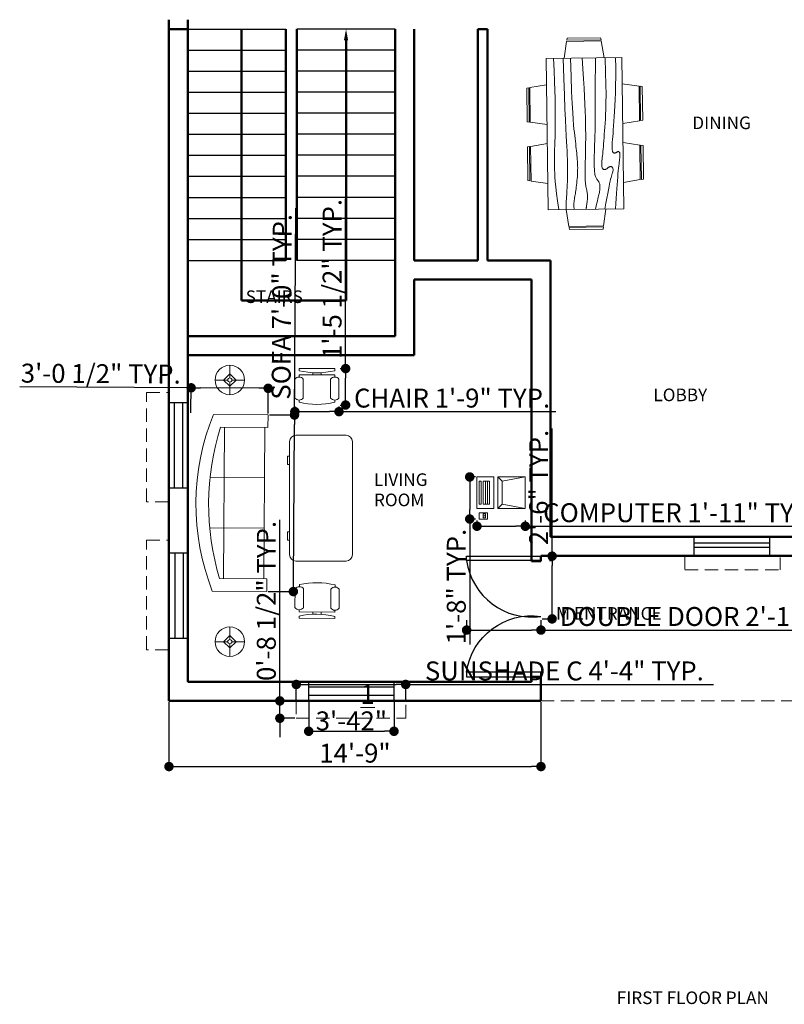
# Model space of a CAD drawing. Units: inches. Extents: x 2050 to 6806, y 2092 to 5743.
# Tile 4 of 8: x 3019 to 3382, y 2203 to 2671. Entities that reach past the tile are written whole.
import ezdxf

# ---------------------------------------------------------------- set-up
doc = ezdxf.new("R2010")
doc.units = ezdxf.units.IN
doc.linetypes.add('HIDDEN', pattern=[9.525, 6.35, -3.175])
for name, color, linetype, lineweight in [('A-ANNO-DIMS', 2, 'Continuous', 18), ('A-ANNO-TEXT', 7, 'Continuous', 25), ('A-AREA-IDEN', 7, 'Continuous', 18), ('A-DOOR', 2, 'Continuous', 25), ('A-FLOR-OVHD', 30, 'HIDDEN', 18), ('A-FLOR-STRS', 3, 'Continuous', 25), ('A-FURN', 5, 'Continuous', 18), ('A-GLAZ', 6, 'Continuous', 25), ('A-WALL', 7, 'Continuous', 50)]:
    doc.layers.add(name, color=color, linetype=linetype, lineweight=lineweight)
doc.styles.get("Standard").update_dxf_attribs({"font": 'arial.ttf'})
doc.dimstyles.new('ISO-25', dxfattribs={"dimtxt": 9, "dimasz": 4.5, "dimexe": 1.25, "dimexo": 0.625, "dimtad": 1, "dimdec": 1, "dimlunit": 4, "dimtxsty": 'Standard', "dimblk": 'DOT', "dimcen": 2.5, "dimadec": 0, "dimazin": 0, "dimtfac": 1, "dimtdec": 1, "dimtmove": 0, "dimatfit": 3, "dimldrblk": 'ARCHTICK', "dimfxl": 1, "dimarcsym": 0})

# ---------------------------------------------------------------- blocks, each defined once
blk = doc.blocks.new('Dining Set - 36 x 72 in.')
for p, q in [((-22.2343, 26.00059), (-23.4847, 17.99762)), ((-22.2304, 26), (-5.7608, 26)), ((-22, 27.5), (-22.1562, 26.50042)), ((-5.8416, 26.5), (-22.1534, 26.5)), ((-22, 27.5), (-6, 27.5)), ((-5.8437, 26.49966), (-6, 27.5)), ((-4.5152, 17.99762), (-5.7655, 25.99926)), ((5.7657, 26.00059), (4.5153, 17.99762)), ((5.7696, 26), (22.2392, 26)), ((6, 27.5), (5.8438, 26.50042)), ((22.1584, 26.5), (5.8466, 26.5)), ((6, 27.5), (22, 27.5)), ((22.1563, 26.49966), (22, 27.5)), ((23.4848, 17.99762), (22.2345, 25.99926)), ((36, 18), (-36, 18)), ((-36, 18), (-36, -18)), ((36, -18), (36, 18)), ((-44.0006, 8.23428), (-35.9976, 9.48474)), ((44.0006, 8.23428), (35.9976, 9.48474)), ((-45.5, 8), (-44.5004, 8.15617)), ((-45.5, 8), (-45.5, -8)), ((-44.5, -8.15843), (-44.5, 8.15338)), ((-44, 8.23041), (-44, -8.23915)), ((44, 8.23041), (44, -8.23915)), ((44.5, -8.15843), (44.5, 8.15338)), ((45.5, 8), (44.5005, 8.15617)), ((45.5, 8), (45.5, -8)), ((-44.4997, -8.15631), (-45.5, -8)), ((-35.9976, -9.48476), (-43.9993, -8.2345)), ((35.9976, -9.48476), (43.9993, -8.2345)), ((44.4997, -8.15631), (45.5, -8)), ((-36, -18), (36, -18)), ((-22.2343, -26.0006), (-23.4847, -17.99762)), ((-4.5152, -17.99762), (-5.7655, -25.99928)), ((5.7657, -26.0006), (4.5153, -17.99762)), ((23.4848, -17.99762), (22.2345, -25.99928)), ((-22.2304, -26), (-5.7608, -26)), ((-22, -27.5), (-22.1562, -26.50044)), ((-5.8416, -26.5), (-22.1534, -26.5)), ((-22, -27.5), (-6, -27.5)), ((-5.8437, -26.49967), (-6, -27.5)), ((5.7696, -26), (22.2392, -26)), ((6, -27.5), (5.8438, -26.50044)), ((22.1584, -26.5), (5.8466, -26.5)), ((6, -27.5), (22, -27.5)), ((22.1563, -26.49967), (22, -27.5))]:
    blk.add_line(p, q)
for points in [[(-36, 15), (-31.1772, 14.97754), (-26.8079, 14.91406), (-22.8538, 14.81543), (-19.276, 14.6875), (-16.0362, 14.53613), (-13.0957, 14.36718), (-10.4159, 14.18652), (-7.9583, 14), (-5.6904, 13.81315), (-3.6035, 13.63021), (-1.6954, 13.45508), (0.0365, 13.29166), (1.5945, 13.14388), (2.9811, 13.01562), (4.1988, 12.9108), (5.25, 12.83333), (6.1393, 12.78613), (6.8802, 12.76823), (7.4883, 12.77767), (7.9792, 12.8125), (8.3685, 12.87077), (8.6719, 12.95052), (8.9049, 13.0498), (9.0833, 13.16666), (9.2205, 13.29899), (9.3216, 13.44401), (9.3895, 13.59879), (9.4271, 13.76041), (9.4373, 13.92594), (9.4232, 14.09245), (9.3875, 14.257), (9.3333, 14.41666), (9.2638, 14.56917), (9.1836, 14.71484), (9.0975, 14.85465), (9.0104, 14.98958), (8.9272, 15.1206), (8.8529, 15.2487), (8.7922, 15.37483), (8.75, 15.5), (8.7305, 15.62467), (8.7344, 15.74739), (8.7617, 15.86621), (8.8125, 15.97916), (8.8867, 16.08431), (8.9844, 16.17968), (9.1055, 16.26334), (9.25, 16.33333), (9.4189, 16.38802), (9.6172, 16.42708), (9.8506, 16.45052), (10.125, 16.45833), (10.4463, 16.45052), (10.8203, 16.42708), (11.2529, 16.38802), (11.75, 16.33333), (12.3184, 16.26318), (12.9694, 16.17838), (13.7151, 16.07991), (14.5677, 15.96875), (15.5395, 15.84586), (16.6426, 15.71224), (17.8893, 15.56884), (19.2917, 15.41666), (20.859, 15.25667), (22.5879, 15.08984), (24.4721, 14.91715), (26.5052, 14.73958), (28.6809, 14.5581), (30.9929, 14.3737), (33.4347, 14.18733), (36, 14)], [(-36, 10), (-28.9766, 10.14274), (-23.1725, 10.20442), (-18.4241, 10.19775), (-14.5677, 10.13541), (-11.4399, 10.03011), (-8.877, 9.89453), (-6.7154, 9.74137), (-4.7917, 9.58333), (-2.9698, 9.43082), (-1.2246, 9.28515), (0.4415, 9.14534), (2.026, 9.01041), (3.5266, 8.87939), (4.9408, 8.7513), (6.266, 8.62516), (7.5, 8.5), (8.6411, 8.37549), (9.6914, 8.2539), (10.6538, 8.13818), (11.5312, 8.03125), (12.3267, 7.93603), (13.043, 7.85547), (13.6831, 7.79248), (14.25, 7.75), (14.7471, 7.7303), (15.1797, 7.73307), (15.5537, 7.75732), (15.875, 7.80208), (16.1494, 7.86637), (16.3828, 7.94922), (16.5811, 8.04964), (16.75, 8.16666), (16.8944, 8.29915), (17.0143, 8.44531), (17.1089, 8.60319), (17.1771, 8.77083), (17.218, 8.94629), (17.2305, 9.1276), (17.2137, 9.31282), (17.1667, 9.5), (17.0895, 9.6875), (16.987, 9.875), (16.8649, 10.0625), (16.7292, 10.25), (16.5856, 10.4375), (16.4401, 10.625), (16.2985, 10.8125), (16.1667, 11), (16.05, 11.18733), (15.9518, 11.3737), (15.8752, 11.5581), (15.8229, 11.73958), (15.798, 11.91715), (15.8034, 12.08984), (15.842, 12.25667), (15.9167, 12.41666), (16.0295, 12.56836), (16.1784, 12.70833), (16.3605, 12.83268), (16.5729, 12.9375), (16.8127, 13.01888), (17.0768, 13.07291), (17.3625, 13.0957), (17.6667, 13.08333), (17.9894, 13.03312), (18.3418, 12.94726), (18.7382, 12.82918), (19.1927, 12.68229), (19.7195, 12.51001), (20.3327, 12.31575), (21.0465, 12.10294), (21.875, 11.875), (22.8357, 11.63354), (23.959, 11.37304), (25.2786, 11.08618), (26.8282, 10.76562), (28.6414, 10.40405), (30.752, 9.99414), (33.1936, 9.52856), (36, 9)], [(-36, 5.5), (-30.7157, 5.3348), (-26.069, 5.20963), (-21.9946, 5.11767), (-18.4271, 5.05208), (-15.3009, 5.00602), (-12.5508, 4.97265), (-10.1112, 4.94515), (-7.9167, 4.91666), (-5.909, 4.88167), (-4.0586, 4.83984), (-2.3429, 4.79215), (-0.7396, 4.73958), (0.7739, 4.6831), (2.22, 4.6237), (3.6213, 4.56233), (5, 4.5), (6.373, 4.43782), (7.7344, 4.3776), (9.0723, 4.32129), (10.375, 4.27083), (11.6309, 4.22819), (12.8281, 4.19531), (13.9551, 4.17415), (15, 4.16666), (15.954, 4.17448), (16.819, 4.19791), (17.6001, 4.23698), (18.3021, 4.29166), (18.9299, 4.36198), (19.4883, 4.44791), (19.9823, 4.54948), (20.4167, 4.66666), (20.7969, 4.79899), (21.1302, 4.94401), (21.4245, 5.09879), (21.6875, 5.26041), (21.9271, 5.42594), (22.1511, 5.59245), (22.3672, 5.757), (22.5834, 5.91666), (22.8065, 6.06868), (23.0404, 6.21093), (23.2879, 6.34147), (23.5521, 6.45833), (23.8358, 6.55957), (24.142, 6.64323), (24.4735, 6.70735), (24.8334, 6.75), (25.2235, 6.76969), (25.642, 6.76692), (26.0858, 6.74267), (26.5521, 6.69791), (27.0379, 6.63362), (27.5404, 6.55078), (28.0565, 6.45036), (28.5834, 6.33333), (29.1242, 6.19987), (29.7071, 6.04687), (30.3661, 5.87044), (31.1354, 5.66666), (32.0493, 5.43164), (33.142, 5.16146), (34.4475, 4.85221), (36, 4.5)], [(-36, -1), (-30.7915, -0.6591), (-26.0195, -0.38216), (-21.6519, -0.16284), (-17.6563, 0.00521), (-14.0005, 0.12833), (-10.6523, 0.21289), (-7.5796, 0.26522), (-4.75, 0.29166), (-2.134, 0.29793), (0.2878, 0.28711), (2.5317, 0.26163), (4.6146, 0.22396), (6.5529, 0.17651), (8.3633, 0.12174), (10.0623, 0.06209), (11.6667, 0), (13.1899, -0.06201), (14.6341, -0.1211), (15.9982, -0.17432), (17.2813, -0.21875), (18.4823, -0.25147), (19.6003, -0.26953), (20.6343, -0.27002), (21.5834, -0.25), (22.4481, -0.20768), (23.2357, -0.14584), (23.9549, -0.06836), (24.6146, 0.02083), (25.2235, 0.11784), (25.7904, 0.21875), (26.3241, 0.31966), (26.8334, 0.41666), (27.3265, 0.50618), (27.8099, 0.58593), (28.2894, 0.65397), (28.7709, 0.70833), (29.2601, 0.74707), (29.763, 0.76823), (30.2855, 0.76985), (30.8334, 0.75), (31.4088, 0.70784), (31.9994, 0.64713), (32.589, 0.57275), (33.1615, 0.48958), (33.7008, 0.4025), (34.1908, 0.3164), (34.6153, 0.23616), (34.9584, 0.16666), (35.2099, 0.11165), (35.3848, 0.07031), (35.504, 0.04069), (35.5886, 0.02083), (35.6594, 0.00879), (35.7377, 0.0026), (35.8442, 0.00032), (36, 0)], [(-36, -6.5), (-27.1843, -6.31267), (-20.084, -6.1263), (-14.469, -5.9419), (-10.1094, -5.76042), (-6.7752, -5.58285), (-4.2363, -5.41016), (-2.2629, -5.24333), (-0.625, -5.08334), (0.8708, -4.93099), (2.2715, -4.78646), (3.5872, -4.64974), (4.8281, -4.52084), (6.0046, -4.39974), (7.127, -4.28646), (8.2053, -4.18099), (9.25, -4.08334), (10.2705, -3.99382), (11.2734, -3.91407), (12.2647, -3.84603), (13.25, -3.79167), (14.2354, -3.75293), (15.2266, -3.73177), (16.2295, -3.73015), (17.25, -3.75), (18.2912, -3.79248), (19.3451, -3.85547), (20.4009, -3.93604), (21.4479, -4.03125), (22.4754, -4.13819), (23.4727, -4.25391), (24.4289, -4.37549), (25.3334, -4.5), (26.1785, -4.62492), (26.9694, -4.74935), (27.7145, -4.87281), (28.4219, -4.99479), (29.1, -5.11483), (29.7572, -5.23242), (30.4016, -5.34709), (31.0417, -5.45834), (31.6837, -5.56437), (32.3262, -5.65821), (32.9658, -5.73153), (33.599, -5.77604), (34.2224, -5.78345), (34.8327, -5.74545), (35.4264, -5.65373), (36, -5.5)], [(-36, -10), (-26.4022, -9.81299), (-18.4675, -9.62891), (-11.9839, -9.45069), (-6.7396, -9.28125), (-2.5226, -9.12354), (0.8789, -8.98047), (3.6769, -8.85498), (6.0833, -8.75), (8.2767, -8.66765), (10.3021, -8.60677), (12.1712, -8.56543), (13.8958, -8.54167), (15.4876, -8.53353), (16.9583, -8.53907), (18.3197, -8.55632), (19.5834, -8.58334), (20.7616, -8.61841), (21.8685, -8.66081), (22.9188, -8.71004), (23.9271, -8.76563), (24.9081, -8.82707), (25.8763, -8.89388), (26.8465, -8.96558), (27.8334, -9.04167), (28.8474, -9.12118), (29.8828, -9.20117), (30.93, -9.27824), (31.9792, -9.34896), (33.0205, -9.40991), (34.0443, -9.45768), (35.0407, -9.48885), (36, -9.5)], [(-36, -14.5), (-30.0881, -14.33513), (-25.0332, -14.21224), (-20.7312, -14.12647), (-17.0781, -14.07292), (-13.97, -14.04671), (-11.3027, -14.04297), (-8.9724, -14.05681), (-6.875, -14.08334), (-4.9224, -14.11833), (-3.0905, -14.16016), (-1.3709, -14.20785), (0.2448, -14.26042), (1.7647, -14.3169), (3.1973, -14.3763), (4.5507, -14.43767), (5.8333, -14.5), (7.0554, -14.5621), (8.235, -14.62175), (9.3922, -14.67652), (10.5469, -14.72396), (11.7192, -14.76164), (12.929, -14.78711), (14.1965, -14.79794), (15.5417, -14.79167), (16.9933, -14.76424), (18.6152, -14.70508), (20.4804, -14.60197), (22.6615, -14.44271), (25.2312, -14.21509), (28.2624, -13.9069), (31.8277, -13.50594), (36, -13)]]:
    blk.add_lwpolyline(points)
blk = doc.blocks.new('Sofa - Roundback 7 ft.')
for p, q in [((-12.00002, -32.4421), (-12.00003, -6.5971)), ((11.99997, -32.4421), (11.99998, -6.5971)), ((-36.000027, -34), (-36.000027, -11.4696)), ((-35.999844, -13.3819), (35.9998, -13.3819)), ((35.99998, -34), (35.99998, -11.4696)), ((-36.000027, -32.4421), (35.99998, -32.4421))]:
    blk.add_line(p, q)
for points in [[(-36.000027, -34), (-42.000027, -34), (-42.000027, -8)], [(41.99998, -8), (41.99998, -34), (35.99998, -34)]]:
    blk.add_lwpolyline(points)
for centre, radius, start, end in [((0, -114.25), 114.25, 68.43141, 111.5686), ((-0.00001, -127.1968), 121.1968, 72.72033, 107.2797)]:
    blk.add_arc(centre, radius, start, end)
blk = doc.blocks.new('Desk - 30 x 60 in.')
for p, q in [((-26.999995, 0), (26.999995, 0)), ((-29.999995, -27), (-29.999995, -3)), ((29.999995, -3), (29.999995, -27)), ((26.999995, -30), (-26.999995, -30)), ((-20.000005, -30), (-20.000005, -31)), ((-20.000005, -31), (-16.000005, -31)), ((-16.000005, -31), (-16.000005, -30)), ((15.999995, -31), (15.999995, -30)), ((19.999995, -31), (15.999995, -31)), ((19.999995, -30), (19.999995, -31))]:
    blk.add_line(p, q)
for centre, start, end in [((-26.499995, -3.5), 98.1301, 171.8699), ((26.499995, -3.5), 8.130102, 81.8699), ((-26.499995, -26.5), 188.1301, 261.8699), ((26.499995, -26.5), 278.1301, 351.8699)]:
    blk.add_arc(centre, 3.535534, start, end)
blk = doc.blocks.new('Chair - Desk')
for p, q in [((-8.5, 0), (-8.5, -1)), ((-8.5, 0), (8.5, 0)), ((8.5, 0), (8.5, -1)), ((-8.5, -3), (-8.5, -4)), ((-8.5, -3), (8.5, -3)), ((-2, -3), (-2, -1.9355)), ((2, -1.9576), (2, -3)), ((8.5, -3), (8.5, -4)), ((-10.5, -5), (-10.5, -14)), ((-6.5, -14), (-6.5, -5)), ((6.5, -5), (6.5, -14)), ((10.5, -14), (10.5, -5)), ((-8.5, -15), (-8.5, -16)), ((8.5, -15), (8.5, -16))]:
    blk.add_line(p, q)
for centre, radius, start, end in [((-8.5, -6.5), 2.5, 36.8699, 143.1301), ((0, 34.625), 36.625, 256.5803, 283.4197), ((8.5, -6.5), 2.5, 36.8699, 143.1301), ((-8.5, -12.5), 2.5, 216.8699, 323.1301), ((8.5, -12.5), 2.5, 216.8699, 323.1301), ((0, 19.625), 36.625, 256.5803, 283.4197)]:
    blk.add_arc(centre, radius, start, end)
blk = doc.blocks.new('Lamp - Table')
for p, q in [((0, 7), (0, 1)), ((-1, 0), (-7, 0)), ((0, 3), (-3, 0)), ((-3, 0), (0, -3)), ((3, 0), (0, 3)), ((0, -3), (3, 0)), ((1, 0), (7, 0)), ((0, -1), (0, -7))]:
    blk.add_line(p, q)
for radius in [7, 1]:
    blk.add_circle((0, 0), radius)
blk = doc.blocks.new('Computer Terminal')
for p, q in [((-10, 11.5), (5, 11.5)), ((-8, 0.5), (-10, 11.5)), ((-10, -1.5), (-10, 11.5)), ((5, 11.5), (3, 0.5)), ((5, 11.5), (5, -1.5)), ((-10, -1.5), (-8, 0.5)), ((3, 0.5), (-8, 0.5)), ((3, 0.5), (5, -1.5)), ((5, -1.5), (-10, -1.5)), ((-10, -11.5), (-10, -3.5)), ((-10, -3.5), (5, -3.5)), ((5, -3.5), (5, -11.5)), ((-8, -5.5), (-8, -8.5)), ((3, -5.5), (-8, -5.5)), ((3, -6.5), (-8, -6.5)), ((-8, -7.5), (3, -7.5)), ((-8, -8.5), (3, -8.5)), ((3, -8.5), (3, -5.5)), ((10, -6.5), (7, -6.5)), ((7, -6.5), (7, -10.5)), ((9.5, -7.5), (7.5, -7.5)), ((7.5, -7.5), (7.5, -8.5)), ((7.5, -8.5), (9.5, -8.5)), ((8.5, -7.5), (8.5, -8.5)), ((9.5, -8.5), (9.5, -7.5)), ((10, -10.5), (10, -6.5)), ((5, -11.5), (-10, -11.5)), ((-8, -9.5), (-8, -10.5)), ((3, -9.5), (-8, -9.5)), ((-8, -10.5), (3, -10.5)), ((3, -10.5), (3, -9.5)), ((7, -10.5), (10, -10.5))]:
    blk.add_line(p, q)
blk = doc.blocks.new('_Dot')
at = {"color": 0, "linetype": 'ByBlock', "lineweight": -2}
blk.add_line((-0.5, 0), (-1, 0), dxfattribs=at)
at = {"color": 0, "linetype": 'ByBlock', "const_width": 0.5}
blk.add_lwpolyline([(-0.25, 0, 1), (0.25, 0, 1)], format="xyb", close=True, dxfattribs=at)
blk = doc.blocks.new('*D41')
at = {"layer": 'A-ANNO-DIMS', "color": 0, "lineweight": -2, "transparency": 16777216}
for p, q in [((3156.16, 2346.7), (3156.16, 2331.62)), ((3196.75, 2346.7), (3196.75, 2331.62)), ((3160.66, 2332.87), (3192.25, 2332.87))]:
    blk.add_line(p, q, dxfattribs=at)
at = {"layer": 'Defpoints', "color": 0, "transparency": 16777216}
for p in [(3156.16, 2347.33), (3196.75, 2347.32), (3196.75, 2332.87)]:
    blk.add_point(p, dxfattribs=at)
at = {"layer": 'A-ANNO-DIMS', "color": 0, "lineweight": -2, "transparency": 16777216, "xscale": 4.5, "yscale": 4.5, "zscale": 4.5, "rotation": 180}
blk.add_blockref('_Dot', (3156.16, 2332.87), dxfattribs=at)
at = {"layer": 'A-ANNO-DIMS', "color": 0, "lineweight": -2, "transparency": 16777216, "xscale": 4.5, "yscale": 4.5, "zscale": 4.5}
blk.add_blockref('_Dot', (3196.75, 2332.87), dxfattribs=at)
at = {"layer": 'A-ANNO-DIMS', "color": 0, "transparency": 16777216, "insert": (3176.46, 2344.12), "char_height": 9, "attachment_point": 5}
blk.add_mtext('3\'-4{\\H1x;\\S1/2;}"', dxfattribs=at)
blk = doc.blocks.new('_ArchTick')
at = {"color": 0, "linetype": 'ByBlock', "const_width": 0.15}
blk.add_lwpolyline([(-0.5, -0.5), (0.5, 0.5)], dxfattribs=at)
blk = doc.blocks.new('*D42')
at = {"layer": 'A-ANNO-DIMS', "color": 0, "lineweight": -2, "transparency": 16777216}
for p, q in [((3089.67, 2346.7), (3089.67, 2314.85)), ((3266.67, 2346.7), (3266.67, 2314.85)), ((3094.17, 2316.1), (3262.17, 2316.1))]:
    blk.add_line(p, q, dxfattribs=at)
at = {"layer": 'Defpoints', "color": 0, "transparency": 16777216}
for p in [(3089.67, 2347.33), (3266.67, 2347.33), (3266.67, 2316.1)]:
    blk.add_point(p, dxfattribs=at)
at = {"layer": 'A-ANNO-DIMS', "color": 0, "lineweight": -2, "transparency": 16777216, "xscale": 4.5, "yscale": 4.5, "zscale": 4.5, "rotation": 180}
blk.add_blockref('_Dot', (3089.67, 2316.1), dxfattribs=at)
at = {"layer": 'A-ANNO-DIMS', "color": 0, "lineweight": -2, "transparency": 16777216, "xscale": 4.5, "yscale": 4.5, "zscale": 4.5}
blk.add_blockref('_Dot', (3266.67, 2316.1), dxfattribs=at)
at = {"layer": 'A-ANNO-DIMS', "color": 0, "transparency": 16777216, "insert": (3178.17, 2321.32), "char_height": 9, "attachment_point": 5}
blk.add_mtext('14\'-9"', dxfattribs=at)
blk = doc.blocks.new('DOOR-750')
blk.add_lwpolyline([(28.97, 0), (26.83, 0), (26.83, 35.38), (28.97, 35.38)], close=True)
blk.add_arc((31.25, 4.42), 31.27, 98.1233, 188.1233)
blk = doc.blocks.new('DOOR-DOUBLE')
blk.add_lwpolyline([(35.38, 28.96), (35.38, 26.82), (0, 26.82), (0, 28.96)], close=True)
blk.add_lwpolyline([(35.38, 28.96), (35.38, 26.82), (0, 26.82), (0, 28.96)], close=True)
blk.add_arc((30.96, 31.24), 31.27, 188.1233, 278.1233)
blk.add_arc((30.96, 31.24), 31.27, 188.1233, 278.1233)
blk = doc.blocks.new('WIN-1050')
for p, q in [((0, 40.58), (9, 40.58)), ((2.5, 0), (2.5, 40.58)), ((6.5, 0), (6.5, 40.58)), ((0, 0), (9, 0))]:
    blk.add_line(p, q)
blk = doc.blocks.new('WIN-900')
for p, q in [((0, 9), (0, 0)), ((36, 5.99), (0, 5.99)), ((36, 9), (36, 0)), ((36, 3.99), (0, 3.99)), ((36, 3.99), (0, 3.99))]:
    blk.add_line(p, q)
blk = doc.blocks.new('SUNSHADE-A')
for p, q in [((0, 52.08), (10.45, 52.08)), ((10.45, 52.08), (10.45, 0)), ((10.45, 0), (0, 0))]:
    blk.add_line(p, q)
blk = doc.blocks.new('SUNSHADE-C')
for p, q in [((0, 8.26), (0, 0)), ((52.07, 0), (52.07, 8.25)), ((0, 0), (52.07, 0))]:
    blk.add_line(p, q)
blk = doc.blocks.new('*D77')
at = {"layer": 'A-ANNO-DIMS', "color": 0, "lineweight": -2, "transparency": 16777216}
for p, q in [((3231.3, 2385.71), (3231.3, 2379.77)), ((3266.67, 2385.71), (3266.67, 2379.77)), ((3235.8, 2381.02), (3262.17, 2381.02)), ((3266.67, 2381.02), (3451.21, 2381.02))]:
    blk.add_line(p, q, dxfattribs=at)
at = {"layer": 'Defpoints', "color": 0, "transparency": 16777216}
for p in [(3231.3, 2386.33), (3266.67, 2386.33), (3266.67, 2381.02)]:
    blk.add_point(p, dxfattribs=at)
at = {"layer": 'A-ANNO-DIMS', "color": 0, "lineweight": -2, "transparency": 16777216, "xscale": 4.5, "yscale": 4.5, "zscale": 4.5, "rotation": 180}
blk.add_blockref('_Dot', (3231.3, 2381.02), dxfattribs=at)
at = {"layer": 'A-ANNO-DIMS', "color": 0, "lineweight": -2, "transparency": 16777216, "xscale": 4.5, "yscale": 4.5, "zscale": 4.5}
blk.add_blockref('_Dot', (3266.67, 2381.02), dxfattribs=at)
at = {"layer": 'A-ANNO-DIMS', "color": 0, "transparency": 16777216, "insert": (3361.19, 2386.31), "char_height": 9, "attachment_point": 5}
blk.add_mtext('DOUBLE DOOR 2\'-11 1/2" TYP.', dxfattribs=at)
blk = doc.blocks.new('*D78')
at = {"layer": 'A-ANNO-DIMS', "color": 0, "lineweight": -2, "transparency": 16777216}
for p, q in [((3271.98, 2416.18), (3271.98, 2476.94)), ((3267.3, 2416.18), (3273.23, 2416.18)), ((3271.98, 2390.83), (3271.98, 2411.68)), ((3267.3, 2386.33), (3273.23, 2386.33))]:
    blk.add_line(p, q, dxfattribs=at)
at = {"layer": 'Defpoints', "color": 0, "transparency": 16777216}
for p in [(3266.67, 2416.18), (3271.98, 2416.18), (3266.67, 2386.33)]:
    blk.add_point(p, dxfattribs=at)
at = {"layer": 'A-ANNO-DIMS', "color": 0, "lineweight": -2, "transparency": 16777216, "xscale": 4.5, "yscale": 4.5, "zscale": 4.5}
for p, rotation in [((3271.98, 2416.18), 90), ((3271.98, 2386.33), 270)]:
    blk.add_blockref('_Dot', p, dxfattribs=dict(at, rotation=rotation))
at = {"layer": 'A-ANNO-DIMS', "color": 0, "transparency": 16777216, "insert": (3266.76, 2448.81), "char_height": 9, "attachment_point": 5, "rotation": 90}
blk.add_mtext('2\'-6" TYP.', dxfattribs=at)
blk = doc.blocks.new('*D83')
at = {"layer": 'A-ANNO-DIMS', "color": 0, "lineweight": -2, "transparency": 16777216}
for p, q in [((3150.25, 2347.95), (3150.25, 2356.39)), ((3202.32, 2347.95), (3202.32, 2356.39)), ((3154.75, 2355.14), (3197.82, 2355.14)), ((3202.32, 2355.14), (3348.82, 2355.14))]:
    blk.add_line(p, q, dxfattribs=at)
at = {"layer": 'Defpoints', "color": 0, "transparency": 16777216}
for p in [(3202.32, 2355.14), (3150.25, 2347.33), (3202.32, 2347.33)]:
    blk.add_point(p, dxfattribs=at)
at = {"layer": 'A-ANNO-DIMS', "color": 0, "lineweight": -2, "transparency": 16777216, "xscale": 4.5, "yscale": 4.5, "zscale": 4.5, "rotation": 180}
blk.add_blockref('_Dot', (3150.25, 2355.14), dxfattribs=at)
at = {"layer": 'A-ANNO-DIMS', "color": 0, "lineweight": -2, "transparency": 16777216, "xscale": 4.5, "yscale": 4.5, "zscale": 4.5}
blk.add_blockref('_Dot', (3202.32, 2355.14), dxfattribs=at)
at = {"layer": 'A-ANNO-DIMS', "color": 0, "transparency": 16777216, "insert": (3277.82, 2360.42), "char_height": 9, "attachment_point": 5}
blk.add_mtext('SUNSHADE C 4\'-4" TYP.', dxfattribs=at)
blk = doc.blocks.new('*D84')
at = {"layer": 'A-ANNO-DIMS', "color": 0, "lineweight": -2, "transparency": 16777216}
for p, q in [((3142.44, 2351.83), (3142.44, 2433.41)), ((3149.63, 2347.33), (3141.19, 2347.33)), ((3142.44, 2339.07), (3142.44, 2347.33)), ((3149.63, 2339.07), (3141.19, 2339.07)), ((3142.44, 2334.57), (3142.44, 2330.07))]:
    blk.add_line(p, q, dxfattribs=at)
at = {"layer": 'Defpoints', "color": 0, "transparency": 16777216}
for p in [(3142.44, 2347.33), (3150.25, 2347.33), (3150.25, 2339.07)]:
    blk.add_point(p, dxfattribs=at)
at = {"layer": 'A-ANNO-DIMS', "color": 0, "lineweight": -2, "transparency": 16777216, "xscale": 4.5, "yscale": 4.5, "zscale": 4.5}
for p, rotation in [((3142.44, 2347.33), 270), ((3142.44, 2339.07), 90)]:
    blk.add_blockref('_Dot', p, dxfattribs=dict(at, rotation=rotation))
at = {"layer": 'A-ANNO-DIMS', "color": 0, "transparency": 16777216, "insert": (3137.16, 2394.87), "char_height": 9, "attachment_point": 5, "rotation": 90}
blk.add_mtext('0\'-8 1/2" TYP.', dxfattribs=at)
blk = doc.blocks.new('*D89')
at = {"layer": 'A-ANNO-DIMS', "color": 0, "lineweight": -2, "transparency": 16777216}
for p, q in [((3149.58, 2487.43), (3149.58, 2483.65)), ((3170.58, 2487.43), (3170.58, 2483.65)), ((3154.08, 2484.9), (3166.08, 2484.9)), ((3170.58, 2484.9), (3273.7, 2484.9))]:
    blk.add_line(p, q, dxfattribs=at)
at = {"layer": 'Defpoints', "color": 0, "transparency": 16777216}
for p in [(3149.58, 2488.05), (3170.58, 2488.05), (3170.58, 2484.9)]:
    blk.add_point(p, dxfattribs=at)
at = {"layer": 'A-ANNO-DIMS', "color": 0, "lineweight": -2, "transparency": 16777216, "xscale": 4.5, "yscale": 4.5, "zscale": 4.5, "rotation": 180}
blk.add_blockref('_Dot', (3149.58, 2484.9), dxfattribs=at)
at = {"layer": 'A-ANNO-DIMS', "color": 0, "lineweight": -2, "transparency": 16777216, "xscale": 4.5, "yscale": 4.5, "zscale": 4.5}
blk.add_blockref('_Dot', (3170.58, 2484.9), dxfattribs=at)
at = {"layer": 'A-ANNO-DIMS', "color": 0, "transparency": 16777216, "insert": (3224.39, 2490.18), "char_height": 9, "attachment_point": 5}
blk.add_mtext('CHAIR 1\'-9" TYP.', dxfattribs=at)
blk = doc.blocks.new('*D90')
at = {"layer": 'A-ANNO-DIMS', "color": 0, "lineweight": -2, "transparency": 16777216}
for p, q in [((3173.73, 2505.38), (3173.73, 2586.12)), ((3171.2, 2505.38), (3174.98, 2505.38)), ((3173.73, 2492.55), (3173.73, 2500.88)), ((3171.2, 2488.05), (3174.98, 2488.05))]:
    blk.add_line(p, q, dxfattribs=at)
at = {"layer": 'Defpoints', "color": 0, "transparency": 16777216}
for p in [(3170.58, 2505.38), (3173.73, 2505.38), (3170.58, 2488.05)]:
    blk.add_point(p, dxfattribs=at)
at = {"layer": 'A-ANNO-DIMS', "color": 0, "lineweight": -2, "transparency": 16777216, "xscale": 4.5, "yscale": 4.5, "zscale": 4.5}
for p, rotation in [((3173.73, 2505.38), 90), ((3173.73, 2488.05), 270)]:
    blk.add_blockref('_Dot', p, dxfattribs=dict(at, rotation=rotation))
at = {"layer": 'A-ANNO-DIMS', "color": 0, "transparency": 16777216, "insert": (3168.45, 2548), "char_height": 9, "attachment_point": 5, "rotation": 90}
blk.add_mtext('1\'-5 1/2" TYP.', dxfattribs=at)
blk = doc.blocks.new('*D95')
at = {"layer": 'A-ANNO-DIMS', "color": 0, "lineweight": -2, "transparency": 16777216}
for p, q in [((3149.41, 2483.32), (3150.05, 2581.61)), ((3137.44, 2483.4), (3150.66, 2483.31)), ((3148.89, 2403.82), (3149.38, 2478.82)), ((3136.89, 2399.4), (3150.11, 2399.32))]:
    blk.add_line(p, q, dxfattribs=at)
at = {"layer": 'Defpoints', "color": 0, "transparency": 16777216}
for p in [(3136.81, 2483.41), (3149.41, 2483.32), (3136.26, 2399.41)]:
    blk.add_point(p, dxfattribs=at)
at = {"layer": 'A-ANNO-DIMS', "color": 0, "lineweight": -2, "transparency": 16777216, "xscale": 4.5, "yscale": 4.5, "zscale": 4.5}
for p, rotation in [((3149.41, 2483.32), 89.62659340575084), ((3148.86, 2399.32), 269.6265934057509)]:
    blk.add_blockref('_Dot', p, dxfattribs=dict(at, rotation=rotation))
at = {"layer": 'A-ANNO-DIMS', "color": 0, "transparency": 16777216, "insert": (3144.46, 2534.75), "char_height": 9, "attachment_point": 5, "rotation": 89.6266}
blk.add_mtext('SOFA 7\'-0" TYP.', dxfattribs=at)
blk = doc.blocks.new('*D96')
at = {"layer": 'A-ANNO-DIMS', "color": 0, "lineweight": -2, "transparency": 16777216}
for p, q in [((3100.23, 2496.24), (3018.65, 2496.78)), ((3100.15, 2484.27), (3100.23, 2497.49)), ((3132.39, 2496.03), (3104.73, 2496.21)), ((3136.81, 2484.03), (3136.9, 2497.25))]:
    blk.add_line(p, q, dxfattribs=at)
at = {"layer": 'Defpoints', "color": 0, "transparency": 16777216}
for p in [(3100.23, 2496.24), (3100.14, 2483.64), (3136.81, 2483.41)]:
    blk.add_point(p, dxfattribs=at)
at = {"layer": 'A-ANNO-DIMS', "color": 0, "lineweight": -2, "transparency": 16777216, "xscale": 4.5, "yscale": 4.5, "zscale": 4.5}
for p, rotation in [((3100.23, 2496.24), 179.6265934057506), ((3136.89, 2496), 359.6265934057507)]:
    blk.add_blockref('_Dot', p, dxfattribs=dict(at, rotation=rotation))
at = {"layer": 'A-ANNO-DIMS', "color": 0, "transparency": 16777216, "insert": (3057.22, 2501.81), "char_height": 9, "attachment_point": 5, "rotation": 359.6266}
blk.add_mtext('3\'-0 1/2" TYP.', dxfattribs=at)
blk = doc.blocks.new('*D99')
at = {"layer": 'A-ANNO-DIMS', "color": 0, "lineweight": -2, "transparency": 16777216}
for p, q in [((3236.22, 2433.21), (3236.22, 2429.14)), ((3259.22, 2433.21), (3259.22, 2429.14)), ((3240.72, 2430.39), (3254.72, 2430.39)), ((3259.22, 2430.39), (3402.15, 2430.39))]:
    blk.add_line(p, q, dxfattribs=at)
at = {"layer": 'Defpoints', "color": 0, "transparency": 16777216}
for p in [(3236.22, 2433.84), (3259.22, 2433.84), (3259.22, 2430.39)]:
    blk.add_point(p, dxfattribs=at)
at = {"layer": 'A-ANNO-DIMS', "color": 0, "lineweight": -2, "transparency": 16777216, "xscale": 4.5, "yscale": 4.5, "zscale": 4.5, "rotation": 180}
blk.add_blockref('_Dot', (3236.22, 2430.39), dxfattribs=at)
at = {"layer": 'A-ANNO-DIMS', "color": 0, "lineweight": -2, "transparency": 16777216, "xscale": 4.5, "yscale": 4.5, "zscale": 4.5}
blk.add_blockref('_Dot', (3259.22, 2430.39), dxfattribs=at)
at = {"layer": 'A-ANNO-DIMS', "color": 0, "transparency": 16777216, "insert": (3332.93, 2435.67), "char_height": 9, "attachment_point": 5}
blk.add_mtext('COMPUTER 1\'-11" TYP.', dxfattribs=at)
blk = doc.blocks.new('*D100')
at = {"layer": 'A-ANNO-DIMS', "color": 0, "lineweight": -2, "transparency": 16777216}
for p, q in [((3235.59, 2453.84), (3231.52, 2453.84)), ((3232.77, 2449.34), (3232.77, 2438.34)), ((3235.59, 2433.84), (3231.52, 2433.84)), ((3232.77, 2433.84), (3232.77, 2374.08))]:
    blk.add_line(p, q, dxfattribs=at)
at = {"layer": 'Defpoints', "color": 0, "transparency": 16777216}
for p in [(3236.22, 2453.84), (3232.77, 2433.84), (3236.22, 2433.84)]:
    blk.add_point(p, dxfattribs=at)
at = {"layer": 'A-ANNO-DIMS', "color": 0, "lineweight": -2, "transparency": 16777216, "xscale": 4.5, "yscale": 4.5, "zscale": 4.5}
for p, rotation in [((3232.77, 2453.84), 90), ((3232.77, 2433.84), 270)]:
    blk.add_blockref('_Dot', p, dxfattribs=dict(at, rotation=rotation))
at = {"layer": 'A-ANNO-DIMS', "color": 0, "transparency": 16777216, "insert": (3227.55, 2401.71), "char_height": 9, "attachment_point": 5, "rotation": 90}
blk.add_mtext('1\'-8" TYP.', dxfattribs=at)

msp = doc.modelspace()

# ---------------------------------------------------------------- linework, layer by layer
at = {"layer": 'A-FLOR-OVHD'}
for p, q in [((3335.17, 2416.33), (3335.17, 2409.73)), ((3380.52, 2409.73), (3380.52, 2415.55)), ((3335.17, 2409.73), (3380.52, 2409.73)), ((3266.67, 2347.33), (3446.67, 2347.33))]:
    msp.add_line(p, q, dxfattribs=at)
at = {"layer": 'A-FLOR-STRS'}
for p, q in [((3098.67, 2666.83), (3134.67, 2666.83)), ((3098.67, 2666.83), (3145.36, 2666.83)), ((3197.28, 2666.83), (3150.59, 2666.83)), ((3197.28, 2666.83), (3161.28, 2666.83)), ((3098.67, 2656.83), (3145.36, 2656.83)), ((3197.28, 2656.83), (3150.59, 2656.83)), ((3098.67, 2646.83), (3145.36, 2646.83)), ((3197.28, 2646.83), (3150.59, 2646.83)), ((3098.67, 2636.83), (3145.36, 2636.83)), ((3197.28, 2636.83), (3150.59, 2636.83)), ((3098.67, 2626.83), (3145.36, 2626.83)), ((3197.28, 2626.83), (3150.59, 2626.83)), ((3098.67, 2616.83), (3145.36, 2616.83)), ((3197.28, 2616.83), (3150.59, 2616.83)), ((3098.67, 2606.83), (3145.36, 2606.83)), ((3197.28, 2606.83), (3150.59, 2606.83)), ((3098.67, 2596.83), (3145.36, 2596.83)), ((3197.28, 2596.83), (3150.59, 2596.83)), ((3098.67, 2586.83), (3145.36, 2586.83)), ((3197.28, 2586.83), (3150.59, 2586.83)), ((3098.67, 2576.83), (3145.36, 2576.83)), ((3197.28, 2576.83), (3150.59, 2576.83)), ((3098.67, 2566.83), (3145.36, 2566.83)), ((3197.28, 2566.83), (3150.59, 2566.83)), ((3098.67, 2556.83), (3145.36, 2556.83)), ((3197.28, 2556.83), (3150.59, 2556.83)), ((3098.67, 2520.83), (3145.36, 2520.83))]:
    msp.add_line(p, q, dxfattribs=at)
at = {"layer": 'A-WALL'}
for p, q in [((3089.67, 2671.33), (3089.67, 2347.33)), ((3098.67, 2671.33), (3098.67, 2356.33)), ((3098.67, 2666.83), (3089.67, 2666.83)), ((3124.15, 2537.84), (3124.15, 2666.83)), ((3145.36, 2666.83), (3145.36, 2556.83)), ((3150.59, 2666.83), (3150.59, 2556.83)), ((3197.28, 2666.83), (3197.28, 2520.83)), ((3206.28, 2666.83), (3206.28, 2556.83)), ((3236.67, 2635.96), (3236.67, 2666.83)), ((3236.67, 2666.83), (3241.17, 2666.83)), ((3241.17, 2635.96), (3241.17, 2666.83)), ((3173.93, 2661.55), (3173.93, 2537.84)), ((3236.67, 2556.83), (3236.67, 2635.96)), ((3241.17, 2556.83), (3241.17, 2635.96)), ((3206.28, 2556.83), (3236.67, 2556.83)), ((3241.17, 2556.83), (3262.17, 2556.83)), ((3262.17, 2556.83), (3271.17, 2556.83)), ((3271.17, 2556.83), (3271.17, 2547.83)), ((3206.28, 2547.83), (3262.17, 2547.83)), ((3206.28, 2547.83), (3206.28, 2511.83)), ((3262.17, 2547.83), (3262.17, 2413.83)), ((3271.17, 2547.83), (3271.17, 2425.33)), ((3173.93, 2537.84), (3124.15, 2537.84)), ((3197.28, 2520.83), (3098.67, 2520.83)), ((3206.28, 2511.83), (3098.67, 2511.83)), ((3271.17, 2425.33), (3442.17, 2425.33)), ((3266.67, 2413.83), (3262.17, 2413.83)), ((3266.67, 2416.33), (3446.67, 2416.33)), ((3266.67, 2416.33), (3266.67, 2413.83)), ((3271.17, 2416.33), (3271.17, 2413.83)), ((3098.67, 2356.33), (3262.17, 2356.33)), ((3262.17, 2358.83), (3262.17, 2356.33)), ((3262.17, 2358.83), (3266.67, 2358.83)), ((3266.67, 2358.83), (3266.67, 2347.33)), ((3089.67, 2347.33), (3266.67, 2347.33))]:
    msp.add_line(p, q, dxfattribs=at)
msp.add_lwpolyline([(3173.93, 2666.83, 0, 2, 0), (3173.93, 2661.55, 2, 2, 0)], format="xyseb", dxfattribs=at)

# ---------------------------------------------------------------- block references
at = {"layer": 'A-DOOR'}
msp.add_blockref('DOOR-DOUBLE', (3231.3, 2387.22), dxfattribs=at)
at = {"layer": 'A-DOOR', "extrusion": (0, 0, -1), "zscale": -1, "rotation": 270}
msp.add_blockref('DOOR-750', (-3266.67, 2387.8), dxfattribs=at)
at = {"layer": 'A-FLOR-OVHD', "rotation": 180}
for p in [(3089.48, 2494.03), (3089.45, 2423.77)]:
    msp.add_blockref('SUNSHADE-A', p, dxfattribs=at)
at = {"layer": 'A-FLOR-OVHD'}
msp.add_blockref('SUNSHADE-C', (3150.25, 2339.07), dxfattribs=at)
at = {"layer": 'A-FURN'}
for name, p, rotation in [('Dining Set - 36 x 72 in.', (3287.66, 2617.14), 270.7337264995932), ('Sofa - Roundback 7 ft.', (3102.54, 2441.63), 89.62659340575055), ('Desk - 30 x 60 in.', (3177, 2443.73), 270), ('Computer Terminal', (3247.72, 2443.84), 270), ('Chair - Desk', (3160.07, 2386.56), 179.3159071844)]:
    msp.add_blockref(name, p, dxfattribs=dict(at, rotation=rotation))
for name, p in [('Lamp - Table', (3118.64, 2499.95)), ('Chair - Desk', (3160.08, 2505.38)), ('Lamp - Table', (3118.64, 2375.49))]:
    msp.add_blockref(name, p, dxfattribs=at)
at = {"layer": 'A-GLAZ'}
for p, rotation in [((3098.68, 2489.07), 180), ((3098.93, 2417.57), 180), ((3196.75, 2347.32), 90.00000000000246)]:
    msp.add_blockref('WIN-1050', p, dxfattribs=dict(at, rotation=rotation))
msp.add_blockref('WIN-900', (3339.43, 2416.33), dxfattribs=at)

# ---------------------------------------------------------------- texts
at = {"layer": 'A-ANNO-TEXT'}
msp.add_text('FIRST FLOOR PLAN', height=6, dxfattribs=at).set_placement((3302.72, 2203.13))
at = {"layer": 'A-AREA-IDEN'}
for s, p in [('DINING', (3338.66, 2619.27)), ('STAIRS', (3126.19, 2536.57)), ('LOBBY', (3320.16, 2489.88)), ('LIVING ', (3187.21, 2449.56)), ('ROOM', (3187.21, 2439.92)), ('M ENTRANCE', (3273.86, 2385.92))]:
    msp.add_text(s, height=6, dxfattribs=at).set_placement(p)

# ---------------------------------------------------------------- dimensions: what is measured, and where the dimension line sits
at = {"layer": 'A-ANNO-DIMS'}
for base, p1, p2, angle, text, picture, middle in [((3173.73, 2505.38), (3170.58, 2488.05), (3170.58, 2505.38), 90, '<> TYP.', '*D90', (3168.45, 2548)), ((3149.41, 2483.32), (3136.26, 2399.41), (3136.81, 2483.41), 89.6266, 'SOFA <> TYP.', '*D95', (3144.46, 2534.75)), ((3100.23, 2496.24), (3136.81, 2483.41), (3100.14, 2483.64), 179.6266, '<> TYP.', '*D96', (3057.22, 2501.81)), ((3271.9778, 2416.1797), (3266.6715, 2386.3313), (3266.6715, 2416.1797), 90, '<> TYP.', '*D78', (3266.7577, 2448.8112)), ((3232.77, 2433.84), (3236.22, 2453.84), (3236.22, 2433.84), 270, '<> TYP.', '*D100', (3227.55, 2401.71)), ((3142.44, 2347.33), (3150.25, 2339.07), (3150.25, 2347.33), 90, '<> TYP.', '*D84', (3137.16, 2394.87))]:
    dim = msp.add_linear_dim(base=base, p1=p1, p2=p2, angle=angle, text=text, dimstyle='ISO-25', override={"dimdec": 1, "dimlfac": 1, "dimrnd": 0, "dimzin": 1, "dimdsep": 46, "dimlunit": 4, "dimfrac": 2}, dxfattribs=at)
    dim.commit()
    dim.dimension.update_dxf_attribs({"geometry": picture, "text_midpoint": middle})
for base, p1, p2, text, picture, middle in [((3170.58, 2484.9), (3149.58, 2488.05), (3170.58, 2488.05), 'CHAIR <> TYP.', '*D89', (3224.39, 2490.18)), ((3259.22, 2430.39), (3236.22, 2433.84), (3259.22, 2433.84), 'COMPUTER <> TYP.', '*D99', (3332.93, 2435.67)), ((3266.67, 2381.02), (3231.3, 2386.33), (3266.67, 2386.33), 'DOUBLE DOOR <> TYP.', '*D77', (3361.19, 2386.31)), ((3202.32, 2355.14), (3150.25, 2347.33), (3202.32, 2347.33), 'SUNSHADE C <> TYP.', '*D83', (3277.82, 2360.42))]:
    dim = msp.add_linear_dim(base=base, p1=p1, p2=p2, text=text, dimstyle='ISO-25', override={"dimdec": 1, "dimlfac": 1, "dimrnd": 0, "dimzin": 1, "dimdsep": 46, "dimlunit": 4, "dimfrac": 2}, dxfattribs=at)
    dim.commit()
    dim.dimension.update_dxf_attribs({"geometry": picture, "text_midpoint": middle})
for base, p1, p2, picture, middle in [((3196.75, 2332.87), (3156.16, 2347.33), (3196.75, 2347.32), '*D41', (3176.46, 2344.12)), ((3266.67, 2316.1), (3089.67, 2347.33), (3266.67, 2347.33), '*D42', (3178.17, 2321.32))]:
    dim = msp.add_linear_dim(base=base, p1=p1, p2=p2, dimstyle='ISO-25', override={"dimclrd": 0, "dimclre": 0, "dimclrt": 0}, dxfattribs=at)
    dim.commit()
    dim.dimension.update_dxf_attribs({"geometry": picture, "text_midpoint": middle})

doc.saveas('drawing.dxf')
